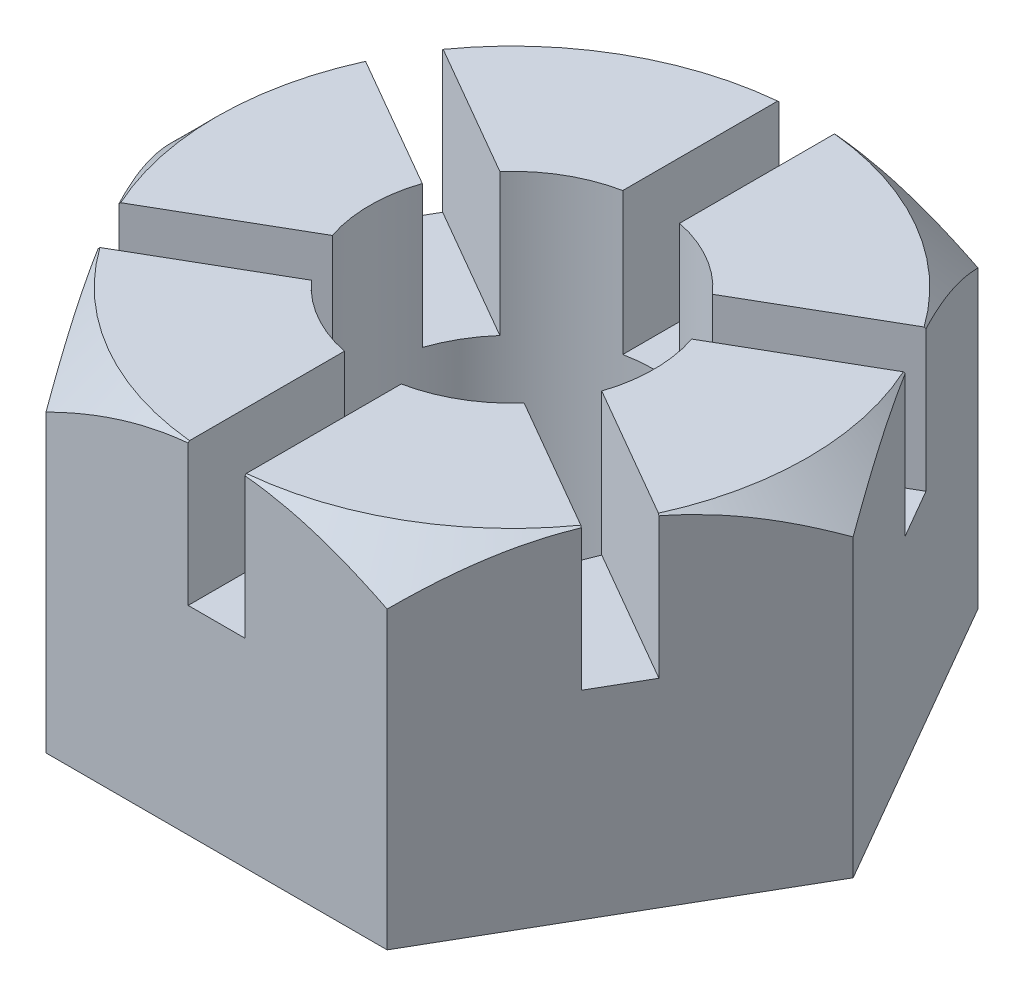
from build123d import *

# Parameters (mm, degrees)
HEX_BODY_104AF_X_60_DEPTH      = 60
CROWN_CHAMFER_SKETCH_OUTSIDE_W = 276.052
CROWN_CHAMFER_SKETCH_OUTSIDE_H = 259.964
CROWN_CHAMFER_SKETCH_OUTSIDE_R = 52
CROWN_CHAMFER_45DEG_DEPTH      = 60
CROWN_CHAMFER_45DEG_DRAFT      = -45
BORE_SKETCH_50_R               = 25
BORE_50_DEPTH                  = 60
CASTLE_SLOTS_6X10_DEPTH        = 25


with BuildPart() as part:
    # Hex Profile Sketch → Hex Body 104AF x 60 (new body)
    with BuildSketch(Plane(origin=(0, 0, 0), x_dir=(1, 0, 0), z_dir=(0, 1, 0))):
        Polygon((30.022213998, -52), (60.044427996, 0), (30.022213998, 52), (-30.022213998, 52), (-60.044427996, 0), (-30.022213998, -52), align=None)
    extrude(amount=HEX_BODY_104AF_X_60_DEPTH)


with BuildPart() as crown_chamfer_45deg_tool:
    # Crown Chamfer Sketch outside → Crown Chamfer 45deg (with draft: the straight prism first)
    with BuildSketch(Plane(origin=(0, 60, 0), x_dir=(1, 0, 0), z_dir=(0, 1, 0))):
        Rectangle(CROWN_CHAMFER_SKETCH_OUTSIDE_W, CROWN_CHAMFER_SKETCH_OUTSIDE_H)
        Circle(CROWN_CHAMFER_SKETCH_OUTSIDE_R, mode=Mode.SUBTRACT)
    extrude(amount=-CROWN_CHAMFER_45DEG_DEPTH)
    # Crown Chamfer 45deg: the draft: its side faces are tilted about the plane it starts from
    crown_chamfer_45deg_sides = [crown_chamfer_45deg_tool.faces().sort_by_distance(p)[0] for p in [
        (0, 30, 129.982),
        (138.026, 30, 0),
        (0, 30, -129.982),
        (-138.026, 30, 0),
        (-52, 30, 0),
    ]]
    draft(crown_chamfer_45deg_sides, Plane(origin=(0, 60, 0), x_dir=(1, 0, 0), z_dir=(0, 1, 0)), CROWN_CHAMFER_45DEG_DRAFT)


with BuildPart() as part_1:
    add(part.part)

    # Crown Chamfer 45deg: cut by crown_chamfer_45deg_tool
    add(crown_chamfer_45deg_tool.part, mode=Mode.SUBTRACT)

    # Bore Sketch Ø50 → Bore Ø50 (cut)
    with BuildSketch(Plane(origin=(0, 60, 0), x_dir=(1, 0, 0), z_dir=(0, 1, 0))):
        with Locations(Location((0, 0, 0), (0, 0, 270))):
            Circle(BORE_SKETCH_50_R)
    extrude(amount=-BORE_50_DEPTH, mode=Mode.SUBTRACT)

    # Castle Slots Sketch → Castle Slots 6x10 (cut)
    with BuildSketch(Plane(origin=(0, 60, 0), x_dir=(1, 0, 0), z_dir=(0, 1, 0))):
        with BuildLine():
            Line((-5, -24.494897428), (-5, -52))
            Line((-5, -52), (0, -52))
            Line((0, -52), (5, -52))
            Line((5, -52), (5, -24.494897428))
            ThreePointArc((5, -24.494897428), (0, -25), (-5, -24.494897428))
        make_face()
        with BuildLine():
            Line((-23.713203436, -7.917321695), (-47.533320997, -21.669872981))
            Line((-47.533320997, -21.669872981), (-45.033320997, -26))
            Line((-45.033320997, -26), (-42.533320997, -30.330127019))
            Line((-42.533320997, -30.330127019), (-18.713203436, -16.577575733))
            ThreePointArc((-18.713203436, -16.577575733), (-21.650635095, -12.5), (-23.713203436, -7.917321695))
        make_face()
        with BuildLine():
            Line((-18.713203436, 16.577575733), (-42.533320997, 30.330127019))
            Line((-42.533320997, 30.330127019), (-45.033320997, 26))
            Line((-45.033320997, 26), (-47.533320997, 21.669872981))
            Line((-47.533320997, 21.669872981), (-23.713203436, 7.917321695))
            ThreePointArc((-23.713203436, 7.917321695), (-21.650635095, 12.5), (-18.713203436, 16.577575733))
        make_face()
        with BuildLine():
            Line((5, 24.494897428), (5, 52))
            Line((5, 52), (0, 52))
            Line((0, 52), (-5, 52))
            Line((-5, 52), (-5, 24.494897428))
            ThreePointArc((-5, 24.494897428), (0, 25), (5, 24.494897428))
        make_face()
        with BuildLine():
            Line((23.713203436, 7.917321695), (47.533320997, 21.669872981))
            Line((47.533320997, 21.669872981), (45.033320997, 26))
            Line((45.033320997, 26), (42.533320997, 30.330127019))
            Line((42.533320997, 30.330127019), (18.713203436, 16.577575733))
            ThreePointArc((18.713203436, 16.577575733), (21.650635095, 12.5), (23.713203436, 7.917321695))
        make_face()
        with BuildLine():
            Line((18.713203436, -16.577575733), (42.533320997, -30.330127019))
            Line((42.533320997, -30.330127019), (45.033320997, -26))
            Line((45.033320997, -26), (47.533320997, -21.669872981))
            Line((47.533320997, -21.669872981), (23.713203436, -7.917321695))
            ThreePointArc((23.713203436, -7.917321695), (21.650635095, -12.5), (18.713203436, -16.577575733))
        make_face()
    extrude(amount=-CASTLE_SLOTS_6X10_DEPTH, mode=Mode.SUBTRACT)


solid = part_1.part
